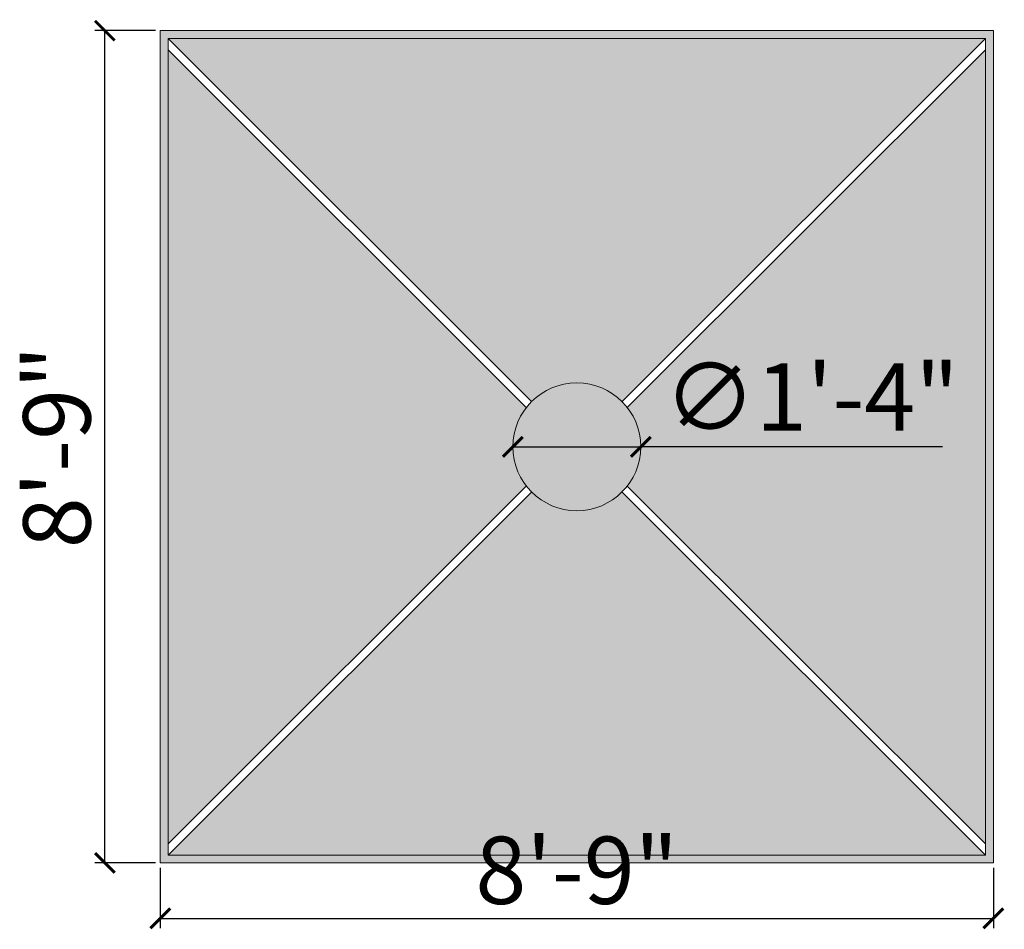
# Model space of a CAD drawing. Units: inches. Extents: x 3799 to 20199, y 1682 to 8087.
# Tile 21 of 30: x 15274 to 15399, y 2711 to 2826. Entities that reach past the tile are written whole.
import ezdxf

# ---------------------------------------------------------------- set-up
doc = ezdxf.new("R2010")
doc.units = ezdxf.units.IN
doc.layers.add('A-ANNO-DIMS', color=2, linetype='Continuous', lineweight=18)
doc.layers.add('A-DETL', color=7, linetype='Continuous', lineweight=18)
doc.styles.get("Standard").update_dxf_attribs({"font": 'arial.ttf'})
doc.dimstyles.new('ISO-25', dxfattribs={"dimtxt": 8.5, "dimasz": 2.5, "dimexe": 1.25, "dimexo": 0.625, "dimtad": 1, "dimdec": 0, "dimlunit": 3, "dimtxsty": 'Standard', "dimblk": 'ARCHTICK', "dimcen": 2.5, "dimadec": 0, "dimazin": 0, "dimtfac": 1, "dimtdec": 0, "dimtmove": 0, "dimatfit": 3, "dimfxl": 1, "dimarcsym": 0})

# ---------------------------------------------------------------- blocks, each defined once
blk = doc.blocks.new('_ArchTick')
at = {"color": 0, "linetype": 'ByBlock', "const_width": 0.15}
blk.add_lwpolyline([(-0.5, -0.5), (0.5, 0.5)], dxfattribs=at)
blk = doc.blocks.new('*D364')
at = {"layer": 'A-ANNO-DIMS', "color": 0, "lineweight": -2, "transparency": 16777216}
for p, q in [((15292.21, 2719.03), (15292.21, 2711.4)), ((15397.4, 2719.03), (15397.4, 2711.4)), ((15292.21, 2712.65), (15397.4, 2712.65))]:
    blk.add_line(p, q, dxfattribs=at)
at = {"layer": 'Defpoints', "color": 0, "transparency": 16777216}
for p in [(15292.21, 2719.65), (15397.4, 2719.65), (15397.4, 2712.65)]:
    blk.add_point(p, dxfattribs=at)
at = {"layer": 'A-ANNO-DIMS', "color": 0, "lineweight": -2, "transparency": 16777216, "xscale": 2.5, "yscale": 2.5, "zscale": 2.5, "rotation": 180}
blk.add_blockref('_ArchTick', (15292.21, 2712.65), dxfattribs=at)
at = {"layer": 'A-ANNO-DIMS', "color": 0, "lineweight": -2, "transparency": 16777216, "xscale": 2.5, "yscale": 2.5, "zscale": 2.5}
blk.add_blockref('_ArchTick', (15397.4, 2712.65), dxfattribs=at)
at = {"layer": 'A-ANNO-DIMS', "color": 0, "transparency": 16777216, "insert": (15344.8, 2717.62), "char_height": 8.5, "attachment_point": 5}
blk.add_mtext('8\'-9"', dxfattribs=at)
blk = doc.blocks.new('*D365')
at = {"layer": 'A-ANNO-DIMS', "color": 0, "lineweight": -2, "transparency": 16777216}
for p, q in [((15291.59, 2824.73), (15283.96, 2824.73)), ((15285.21, 2719.65), (15285.21, 2824.73)), ((15291.59, 2719.65), (15283.96, 2719.65))]:
    blk.add_line(p, q, dxfattribs=at)
at = {"layer": 'Defpoints', "color": 0, "transparency": 16777216}
for p in [(15285.21, 2824.73), (15292.21, 2824.73), (15292.21, 2719.65)]:
    blk.add_point(p, dxfattribs=at)
at = {"layer": 'A-ANNO-DIMS', "color": 0, "lineweight": -2, "transparency": 16777216, "xscale": 2.5, "yscale": 2.5, "zscale": 2.5}
for p, rotation in [((15285.21, 2824.73), 90), ((15285.21, 2719.65), 270)]:
    blk.add_blockref('_ArchTick', p, dxfattribs=dict(at, rotation=rotation))
at = {"layer": 'A-ANNO-DIMS', "color": 0, "transparency": 16777216, "insert": (15280.25, 2772.19), "char_height": 8.5, "attachment_point": 5, "rotation": 90}
blk.add_mtext('8\'-9"', dxfattribs=at)
blk = doc.blocks.new('*D384')
at = {"layer": 'A-ANNO-DIMS', "color": 0, "lineweight": -2, "transparency": 16777216}
for p in [(15336.73, 2772.19), (15390.97, 2772.19)]:
    blk.add_line(p, (15352.88, 2772.19), dxfattribs=at)
at = {"layer": 'Defpoints', "color": 0, "transparency": 16777216}
for p in [(15336.73, 2772.19), (15352.88, 2772.19)]:
    blk.add_point(p, dxfattribs=at)
at = {"layer": 'A-ANNO-DIMS', "color": 0, "lineweight": -2, "transparency": 16777216, "xscale": 2.5, "yscale": 2.5, "zscale": 2.5}
for p, rotation in [((15336.73, 2772.19), 0.00106432091596), ((15352.88, 2772.19), 180.0010643209159)]:
    blk.add_blockref('_ArchTick', p, dxfattribs=dict(at, rotation=rotation))
at = {"layer": 'A-ANNO-DIMS', "color": 0, "transparency": 16777216, "insert": (15374.43, 2777.39), "char_height": 8.5, "attachment_point": 5, "rotation": 0.0011}
blk.add_mtext('∅1\'-4"', dxfattribs=at)

msp = doc.modelspace()

# ---------------------------------------------------------------- hatches: boundary and pattern name
at = {"layer": 'A-DETL'}
h = msp.add_hatch(color=256, dxfattribs=at)
h.dxf.hatch_style = 1
h.paths.add_polyline_path([(15292.21, 2824.73), (15292.21, 2719.65), (15397.4, 2719.65), (15397.4, 2824.73)])
h.paths.add_polyline_path([(15293.21, 2823.73), (15293.21, 2720.65), (15396.4, 2720.65), (15396.4, 2823.73)], flags=16)
h.paths.add_polyline_path([(15352.88, 2772.19, -1), (15336.73, 2772.19, -1)], flags=0)
h = msp.add_hatch(color=256, dxfattribs=at)
h.dxf.hatch_style = 1
h.set_gradient(color1=(229, 232, 120), color2=(122, 175, 223), name='SPHERICAL')
h.paths.add_polyline_path([(15293.21, 2823.73), (15339.09, 2777.9, -0.414518), (15350.52, 2777.9), (15396.4, 2823.73)])
h = msp.add_hatch(color=256, dxfattribs=at)
h.dxf.hatch_style = 1
h.set_gradient(color1=(88, 186, 72), color2=(206, 204, 230), name='SPHERICAL')
h.paths.add_polyline_path([(15338.43, 2767.24, -0.166699), (15336.73, 2772.19, -0.166699), (15338.43, 2777.15), (15293.21, 2822.32), (15293.21, 2722.07)])
h.paths.add_polyline_path([(15396.4, 2722.07), (15396.4, 2822.32), (15351.18, 2777.15, -0.166699), (15352.88, 2772.19, -0.166699), (15351.18, 2767.24)])
h = msp.add_hatch(color=256, dxfattribs=at)
h.dxf.hatch_style = 1
h.paths.add_polyline_path([(15352.88, 2772.19, 1), (15336.73, 2772.19, 1)])
h = msp.add_hatch(color=256, dxfattribs=at)
h.dxf.hatch_style = 1
h.set_gradient(color1=(88, 186, 72), color2=(19, 155, 72), name='SPHERICAL')
h.paths.add_polyline_path([(15396.4, 2720.65), (15350.52, 2766.48, -0.414518), (15339.09, 2766.48), (15293.21, 2720.65)])

# ---------------------------------------------------------------- linework, layer by layer
for p, q in [((15292.21, 2824.73), (15397.4, 2824.73)), ((15292.21, 2719.65), (15292.21, 2824.73)), ((15397.4, 2824.73), (15397.4, 2719.65)), ((15339.09, 2777.9), (15293.21, 2823.73)), ((15293.21, 2823.73), (15396.4, 2823.73)), ((15293.21, 2720.65), (15293.21, 2823.73)), ((15350.52, 2777.9), (15396.4, 2823.73)), ((15396.4, 2823.73), (15396.4, 2720.65)), ((15338.38, 2777.19), (15293.21, 2822.32)), ((15351.22, 2777.19), (15396.4, 2822.32)), ((15293.21, 2722.07), (15338.38, 2767.19)), ((15293.21, 2720.65), (15339.09, 2766.48)), ((15396.4, 2720.65), (15350.52, 2766.48)), ((15396.4, 2722.07), (15351.22, 2767.19)), ((15396.4, 2720.65), (15293.21, 2720.65)), ((15397.4, 2719.65), (15292.21, 2719.65))]:
    msp.add_line(p, q, dxfattribs=at)
msp.add_circle((15344.8, 2772.19), 8.07, dxfattribs=at)

# ---------------------------------------------------------------- dimensions: what is measured, and where the dimension line sits
at = {"layer": 'A-ANNO-DIMS'}
dim = msp.add_linear_dim(base=(15285.21, 2824.73), p1=(15292.21, 2719.65), p2=(15292.21, 2824.73), angle=90, dimstyle='ISO-25', override={"dimdec": 1, "dimlfac": 1, "dimrnd": 0, "dimzin": 1, "dimdsep": 46, "dimlunit": 4, "dimfrac": 2}, dxfattribs=at)
dim.commit()
dim.dimension.update_dxf_attribs({"geometry": '*D365', "text_midpoint": (15280.25, 2772.19)})
dim = msp.add_diameter_dim_2p(p1=(15336.72942, 2772.1917), p2=(15352.87937, 2772.192), dimstyle='ISO-25', override={"dimdec": 1, "dimlfac": 1, "dimrnd": 0, "dimzin": 1, "dimdsep": 46, "dimlunit": 4, "dimfrac": 2}, dxfattribs=at)
dim.commit()
dim.dimension.update_dxf_attribs({"geometry": '*D384', "text_midpoint": (15374.42593, 2772.1924), "dimtype": 163})
dim = msp.add_linear_dim(base=(15397.4, 2712.65), p1=(15292.21, 2719.65), p2=(15397.4, 2719.65), dimstyle='ISO-25', override={"dimdec": 1, "dimlfac": 1, "dimrnd": 0, "dimzin": 1, "dimdsep": 46, "dimlunit": 4, "dimfrac": 2}, dxfattribs=at)
dim.commit()
dim.dimension.update_dxf_attribs({"geometry": '*D364', "text_midpoint": (15344.8, 2717.62)})

doc.saveas('drawing.dxf')
